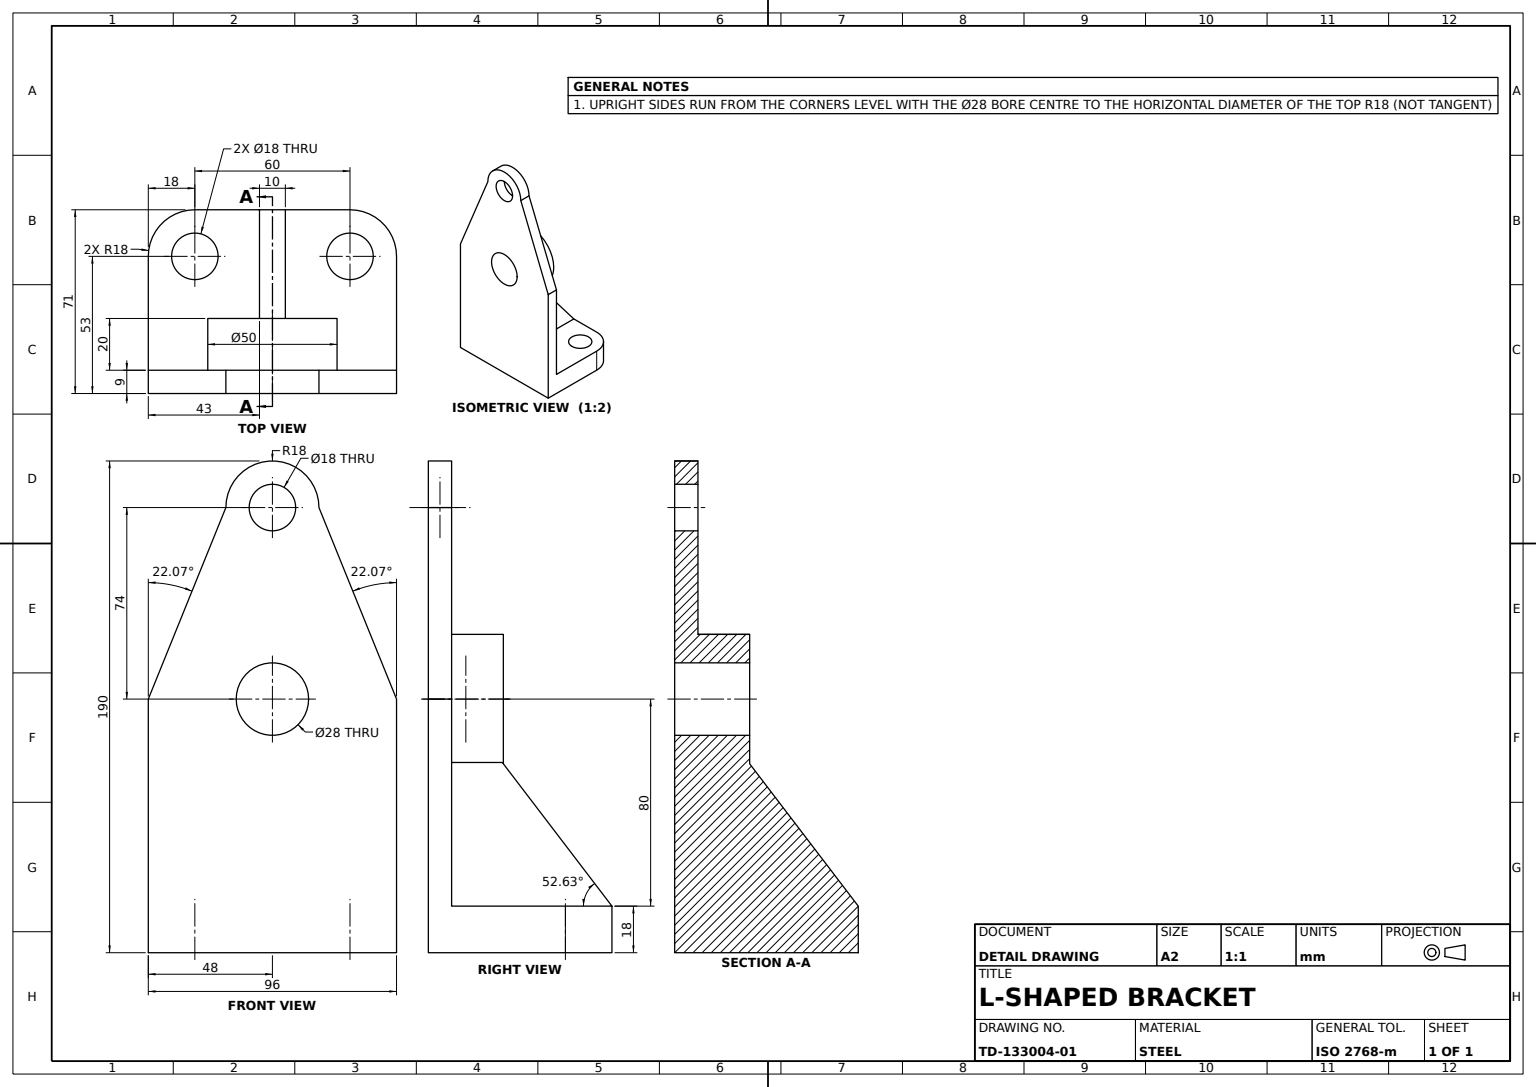
SolidWorks part; units mm, degrees
material "Plain Carbon Steel"
ref_plane "Front Plane" through (0, 0, 0) normal (0, 0, 1) x (1, 0, 0)
ref_plane "Top Plane" through (0, 0, 0) normal (0, 1, 0) x (1, 0, 0)
ref_plane "Right Plane" through (0, 0, 0) normal (1, 0, 0) x (0, 0, -1)
sketch "Base Plate Sketch" plane through (0, 0, 0) normal (0, 1, 0) x (1, 0, 0)
  line L0 (0, 0) -> (0, 53)
  line L1 (18, 71) -> (78, 71)
  line L2 (96, 53) -> (96, 0)
  line L3 (96, 0) -> (0, 0)
  arc A0 (0, 53) -> (18, 71) centre (18, 53) cw
  arc A1 (78, 71) -> (96, 53) centre (78, 53) cw
  dimension "D1" = 18
  dimension "D2" = 18
  dimension "D3" = 96
  dimension "D4" = 60
  dimension "D5" = 53
extrude "Base Plate" add sketch "Base Plate Sketch" along normal blind 18
sketch "Upright Plate Sketch" plane through (0, 0, 0) normal (0, 0, 1) x (1, 0, 0)
  line L0 (0, 18) -> (0, 98)
  line L1 (48, 18) -> (48, 172) construction
  line L2 (0, 18) -> (96, 18) construction
  line L3 (30, 172) -> (0, 98)
  line L4 (66, 172) -> (96, 98)
  line L5 (96, 98) -> (96, 18)
  line L6 (30, 172) -> (66, 172)
  line L7 (96, 18) -> (0, 18)
  circle A0 centre (48, 172) radius 18
  circle A1 centre (48, 172) radius 9
  line M10 (96, 18) -> (0, 18)
  dimension "D3" = 36
  dimension "D4" = 18
  dimension "D1" = 80
  dimension "D2" = 154
  dimension "D5" = 74
extrude "Upright Plate" add sketch "Upright Plate Sketch" against normal blind 9 contours L1 L5 L4 A0 M10 | L7 L1 A0 L3 L0 | A0 L1 A1 L6
sketch "Upright Top Hole Sketch" plane through (0, 0, -9) normal (0, 0, -1) x (-1, 0, 0)
  circle A0 centre (-48, 172) radius 9
  dimension "D1" = 18
extrude "Upright Top Hole Ø18" cut sketch "Upright Top Hole Sketch" against normal blind 9
sketch "Hub Boss Sketch" plane through (0, 0, -9) normal (0, 0, -1) x (-1, 0, 0)
  line L0 (-96, 98) -> (0, 98) construction
  circle A0 centre (-48, 98) radius 25
  dimension "D1" = 50
extrude "Hub Boss" add sketch "Hub Boss Sketch" along normal blind 20
sketch "Hub Bore Sketch" plane through (0, 0, -29) normal (0, 0, -1) x (-1, 0, 0)
  circle A0 centre (-48, 98) radius 14
  dimension "D1" = 28
extrude "Hub Bore Ø28" cut sketch "Hub Bore Sketch" against normal through all
sketch "Base Hole Sketch" plane through (0, 0, 0) normal (0, -1, 0) x (1, 0, 0)
  circle A0 centre (18, -53) radius 9
  circle A1 centre (78, -53) radius 9
  dimension "D1" = 18
  dimension "D2" = 18
extrude "Base Hole Ø18" cut sketch "Base Hole Sketch" against normal through all
ref_plane "Rib Mid Plane" through (48, 0, 0) normal (1, 0, 0) x (0, 0, -1)
sketch "Support Rib Sketch" plane through (48, 0, 0) normal (1, 0, 0) x (0, 0, -1)
  line L0 (29, 73) -> (71, 18)
rib "Support Rib" sketch "Support Rib Sketch" sketch "Support Rib Sketch" thickness 10 extrusion direction parallel to sketch draft on no parameters "D1"=10
